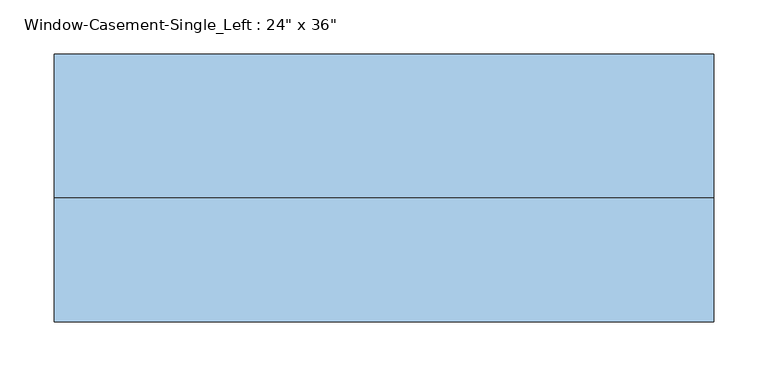
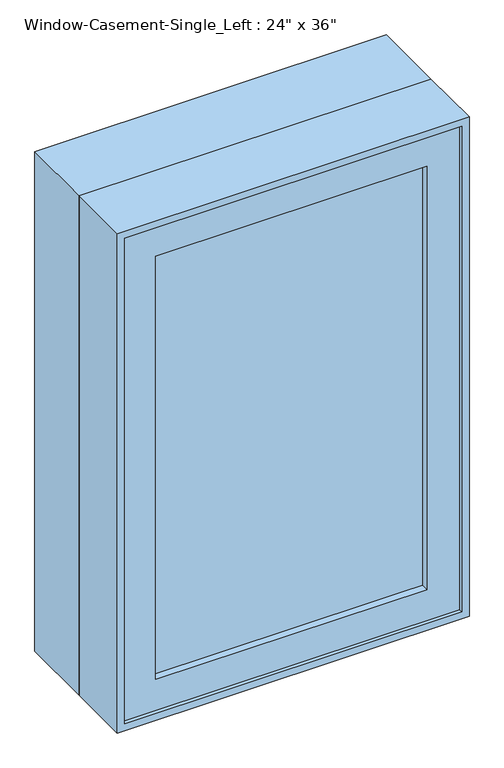
"""IFC4 building model written with IfcOpenShell, lengths in millimetres: window geometry."""

from ifc_helpers import new_model, si_unit, frame, origin, place, context, project, spatial, polyline, outline, extrude, faceted_brep, source, transform, mapped, element, save


def window_25e7c868(model_context):
    return source(origin(), model_context, "Body", "SolidModel", [
        faceted_brep([(273.05, -82.55, 1797.05), (-273.05, -82.55, 1797.05), (-273.05, -19.05, 1797.05), (273.05, -19.05, 1797.05), (292.1, -133.35, 1816.1), (-292.1, -133.35, 1816.1), (-292.1, -82.55, 1816.1), (292.1, -82.55, 1816.1), (304.8, -19.05, 1828.8), (-304.8, -19.05, 1828.8), (-304.8, -133.35, 1828.8), (304.8, -133.35, 1828.8), (-273.05, -82.55, 946.15), (-273.05, -19.05, 946.15), (-292.1, -133.35, 927.1), (-292.1, -82.55, 927.1), (-304.8, -19.05, 914.4), (-304.8, -133.35, 914.4), (273.05, -82.55, 946.15), (273.05, -19.05, 946.15), (292.1, -133.35, 927.1), (292.1, -82.55, 927.1), (304.8, -19.05, 914.4), (304.8, -133.35, 914.4)], [[[0, 1, 2, 3]], [[4, 5, 6, 7]], [[8, 9, 10, 11]], [[1, 12, 13, 2]], [[5, 14, 15, 6]], [[9, 16, 17, 10]], [[12, 18, 19, 13]], [[14, 20, 21, 15]], [[16, 22, 23, 17]], [[9, 8, 22, 16], [3, 2, 13, 19]], [[18, 0, 3, 19]], [[7, 6, 15, 21], [1, 0, 18, 12]], [[20, 4, 7, 21]], [[22, 8, 11, 23]], [[11, 10, 17, 23], [5, 4, 20, 14]]]),
        extrude(outline(polyline([(1828.8, -304.8), (914.4, -304.8), (914.4, 304.8), (1828.8, 304.8), (1828.8, -304.8)]), holes=[polyline([(1809.75, 285.75), (933.45, 285.75), (933.45, -285.75), (1809.75, -285.75), (1809.75, 285.75)])]), frame((0.0, -19.05, 0.0), z_axis=(0.0, 1.0, 0.0), x_axis=(0.0, 0.0, 1.0)), (0.0, 0.0, 1.0), 133.35),
        extrude(outline(polyline([(1816.1, 292.1), (1816.1, -292.1), (927.1, -292.1), (927.1, 292.1), (1816.1, 292.1)]), holes=[polyline([(1758.95, -234.95), (1758.95, 234.95), (984.25, 234.95), (984.25, -234.95), (1758.95, -234.95)])]), frame((0.0, -127.0, 0.0), z_axis=(0.0, 1.0, 0.0), x_axis=(0.0, 0.0, 1.0)), (0.0, 0.0, 1.0), 44.45),
        extrude(outline(polyline([(234.95, -114.3), (-234.95, -114.3), (-234.95, -107.95), (234.95, -107.95), (234.95, -114.3)])), frame((0.0, 0.0, 984.25), z_axis=(0.0, 0.0, 1.0), x_axis=(1.0, 0.0, 0.0)), (0.0, 0.0, 1.0), 774.7),
        extrude(outline(polyline([(-234.95, -95.25), (234.95, -95.25), (234.95, -101.6), (-234.95, -101.6), (-234.95, -95.25)])), frame((0.0, 0.0, 984.25), z_axis=(0.0, 0.0, 1.0), x_axis=(1.0, 0.0, 0.0)), (0.0, 0.0, 1.0), 774.7),
    ])


if __name__ == "__main__":
    model = new_model("IFC4")
    model_context = context("Model", 3, world=origin())
    ifc_project = project(units=[si_unit("LENGTHUNIT", "METRE", prefix="MILLI")], contexts=[model_context])
    site = spatial("IfcSite", under=ifc_project)
    building = spatial("IfcBuilding", under=site)
    placement = place(None, origin())
    window_shape = window_25e7c868(model_context)
    element("IfcWindow", 1, ObjectType="Window-Casement-Single_Left : 24\" x 36\"", at=placement, inside=building, context=model_context, shape_type="MappedRepresentation", body=[
        mapped(window_shape, transform((0.0, 0.0, 0.0), x_axis=(1.0, 0.0, 0.0), y_axis=(0.0, 1.0, 0.0), z_axis=(0.0, 0.0, 1.0))),
    ])
    save(model, "model.ifc")

# Revit data of these elements
# Type "Window-Casement-Single_Left : 24\" x 36\""
#   Type Mark = "18"
#   Fire Rating = "0.5h"
#   Assembly Code = "B2020100"
#   Analytic Construction = "Double glazing - domestic"
#   Window Inset [instance default] = 0' - 0"
#   Wall Thickness [instance default] = 0' - 6"
#   Visual Light Transmittance = 0.81
#   Thermal Resistance (R) = 1.8146 (h·ft²·°F)/BTU
#   Solar Heat Gain Coefficient = 0.76
#   Rough Width = 2' - 0 1/2"
#   Rough Height = 3' - 0 1/2"
#   Interior Wall Closure [instance default] = 0' - 2 1/4"
#   Height = 3' - 0"
#   Heat Transfer Coefficient (U) = 0.5511 BTU/(h·ft²·°F)
#   Frame Extension [instance default] = 0' - 0 1/4"
#   Exterior Wall Closure [instance default] = 0' - 1 1/4"
#   Extension Jamb [instance default] = 0' - 2 1/4"
#   Default Sill Height = 3' - 0"
#   Width = 2' - 0"
#   Muntin Visibility = yes
#   Interior Trim Visibility [instance default] = yes
#   Exterior Trim Visibility [instance default] = yes
#   Extension Jamb Visibility [instance default] = yes
#   Muntin Pattern = Muntin Pattern_2x2 : Muntin Pattern_2x2
#   Interior Trim Material = Wood - Stained
#   Interior Trim = Trim-Window-Interior-Flat : Picture Frame
#   Interior Frame Material = Wood - Stained
#   Glass Panel Material = Glass
#   Exterior Trim Material = Clad - White
#   Exterior Trim = Trim-Window-Exterior-Flat : with Sill
#   Exterior Frame Material = Clad - White
#   Wall Closure = (empty or 0)
# Element 1 (IfcWindow, "Window-Casement-Single_Left : 24\" x 36\"")
#   Wall Thickness = 0' - 9"
#   Extension Jamb = 0' - 5 1/4"
#   Materials on its faces: "Wood - Stained", "Glass", "Clad - White"
# Materials
#   "Wood - Stained": class "Wood", colour RGB 224 178 126, transparency 0, Cost = 0
#   "Glass": class "Glass", colour RGB 0 128 192, transparency 0.75, Description = "Soda Lime Glass", Cost = 0
#   "Clad - White": class "Wood", colour RGB 242 242 238, transparency 0, Cost = 0
